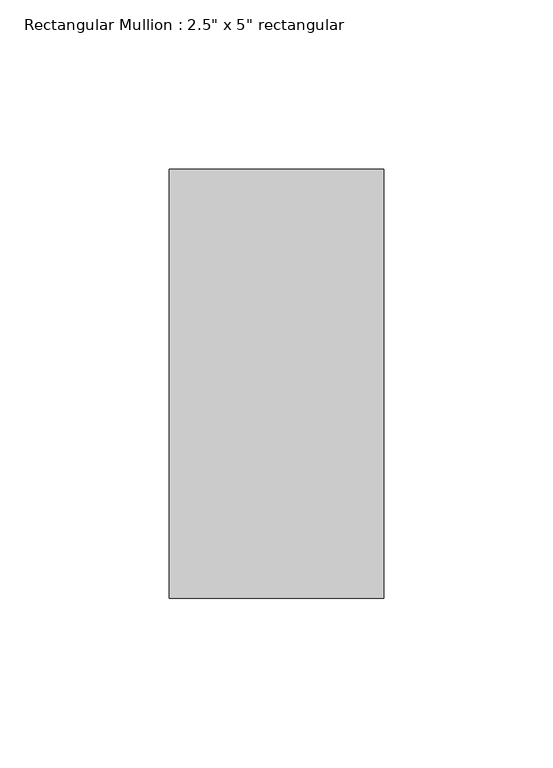
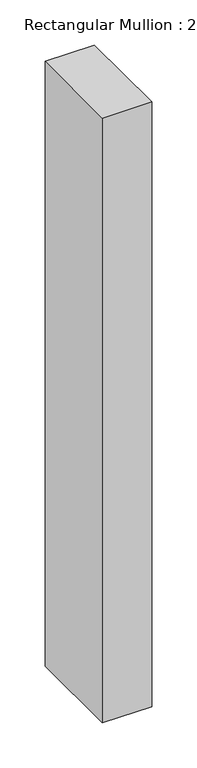
"""IFC4 building model written with IfcOpenShell, lengths in millimetres: member geometry."""

from ifc_helpers import new_model, si_unit, frame, origin, place, context, project, spatial, polyline, outline, extrude, source, transform, mapped, element, save


def member_63078a24(model_context):
    return source(origin(), model_context, "Body", "SweptSolid", [
        extrude(outline(polyline([(0.0, 63.5), (0.0, -63.5), (-63.5, -63.5), (-63.5, 63.5), (0.0, 63.5)])), frame((0.0, 0.0, -820.3881029), z_axis=(0.0, 0.0, 1.0), x_axis=(1.0, 0.0, 0.0)), (0.0, 0.0, 1.0), 820.3881029),
    ])


if __name__ == "__main__":
    model = new_model("IFC4")
    model_context = context("Model", 3, world=origin())
    ifc_project = project(units=[si_unit("LENGTHUNIT", "METRE", prefix="MILLI")], contexts=[model_context])
    site = spatial("IfcSite", under=ifc_project)
    building = spatial("IfcBuilding", under=site)
    placement = place(None, origin())
    member_shape = member_63078a24(model_context)
    element("IfcMember", 1, ObjectType="Rectangular Mullion : 2.5\" x 5\" rectangular", at=placement, inside=building, context=model_context, shape_type="MappedRepresentation", body=[
        mapped(member_shape, transform((0.0, 0.0, 0.0), x_axis=(1.0, 0.0, 0.0), y_axis=(0.0, 1.0, 0.0), z_axis=(0.0, 0.0, 1.0))),
    ])
    save(model, "model.ifc")

# Revit data of these elements
# Type "Rectangular Mullion : 2.5\" x 5\" rectangular"
#   built-in parameter 1007304 = 0.416667 (stored number, unit not read)
#   built-in parameter 1007301 = 0.104167 (stored number, unit not read)
#   built-in parameter 1007300 = 0.104167 (stored number, unit not read)
# Element 1 (IfcMember, "Rectangular Mullion : 2.5\" x 5\" rectangular")
#   Materials on its faces: "Aluminum"
# Materials
#   "Aluminum": class "Metal", colour RGB 247 247 247, transparency 0, Description = "Aluminum 6061", Cost = 0
